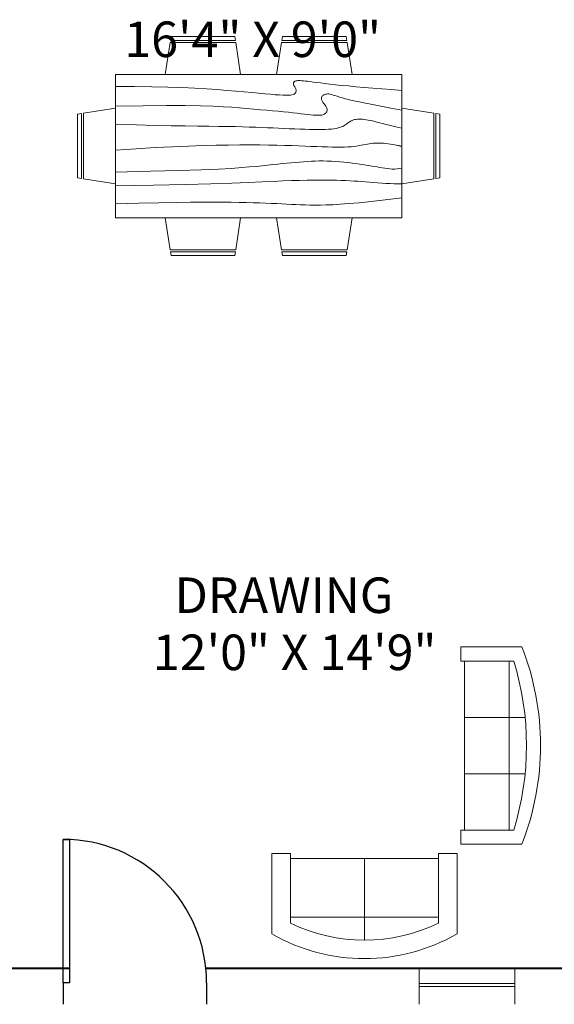
# Model space of a CAD drawing. Units: inches. Extents: x -46 to 1145, y -527 to 760.
# Tile 55 of 57: x 775 to 909, y 222 to 469. Entities that reach past the tile are written whole.
import ezdxf

# ---------------------------------------------------------------- set-up
doc = ezdxf.new("R2010")
doc.units = ezdxf.units.IN
doc.header["$MEASUREMENT"] = 0
for name, color, linetype, lineweight in [('A-AREA-IDEN', 1, 'Continuous', 18), ('A-FURN', 2, 'Continuous', 13), ('DOORS', 3, 'Continuous', 25), ('WALLS', 4, 'Continuous', 40), ('WINDOWS', 240, 'Continuous', 20)]:
    doc.layers.add(name, color=color, linetype=linetype, lineweight=lineweight)
doc.styles.get("Standard").update_dxf_attribs({"font": 'arial.ttf'})

# ---------------------------------------------------------------- blocks, each defined once
blk = doc.blocks.new('Dining Set - 36 x 72 in.')
for p, q in [((-22, 27.5), (-22.1562, 26.50042)), ((-22, 27.5), (-6, 27.5)), ((-5.8437, 26.49966), (-6, 27.5)), ((6, 27.5), (5.8438, 26.50042)), ((6, 27.5), (22, 27.5)), ((22.1563, 26.49966), (22, 27.5)), ((-22.2343, 26.00059), (-23.4847, 17.99762)), ((-22.2304, 26), (-5.7608, 26)), ((-5.8416, 26.5), (-22.1534, 26.5)), ((-4.5152, 17.99762), (-5.7655, 25.99926)), ((5.7657, 26.00059), (4.5153, 17.99762)), ((5.7696, 26), (22.2392, 26)), ((22.1584, 26.5), (5.8466, 26.5)), ((23.4848, 17.99762), (22.2345, 25.99926)), ((36, 18), (-36, 18)), ((-36, 18), (-36, -18)), ((36, -18), (36, 18)), ((-45.5, 8), (-44.5004, 8.15617)), ((-45.5, 8), (-45.5, -8)), ((-44.5, -8.15843), (-44.5, 8.15338)), ((-44.0006, 8.23428), (-35.9976, 9.48474)), ((-44, 8.23041), (-44, -8.23915)), ((44.0006, 8.23428), (35.9976, 9.48474)), ((44, 8.23041), (44, -8.23915)), ((44.5, -8.15843), (44.5, 8.15338)), ((45.5, 8), (44.5005, 8.15617)), ((45.5, 8), (45.5, -8)), ((-44.4997, -8.15631), (-45.5, -8)), ((-35.9976, -9.48476), (-43.9993, -8.2345)), ((35.9976, -9.48476), (43.9993, -8.2345)), ((44.4997, -8.15631), (45.5, -8)), ((-36, -18), (36, -18)), ((-22.2343, -26.0006), (-23.4847, -17.99762)), ((-4.5152, -17.99762), (-5.7655, -25.99928)), ((5.7657, -26.0006), (4.5153, -17.99762)), ((23.4848, -17.99762), (22.2345, -25.99928)), ((-22.2304, -26), (-5.7608, -26)), ((-22, -27.5), (-22.1562, -26.50044)), ((-5.8416, -26.5), (-22.1534, -26.5)), ((-5.8437, -26.49967), (-6, -27.5)), ((5.7696, -26), (22.2392, -26)), ((6, -27.5), (5.8438, -26.50044)), ((22.1584, -26.5), (5.8466, -26.5)), ((22.1563, -26.49967), (22, -27.5)), ((-22, -27.5), (-6, -27.5)), ((6, -27.5), (22, -27.5))]:
    blk.add_line(p, q)
for points in [[(-36, 15), (-31.1772, 14.97754), (-26.8079, 14.91406), (-22.8538, 14.81543), (-19.276, 14.6875), (-16.0362, 14.53613), (-13.0957, 14.36718), (-10.4159, 14.18652), (-7.9583, 14), (-5.6904, 13.81315), (-3.6035, 13.63021), (-1.6954, 13.45508), (0.0365, 13.29166), (1.5945, 13.14388), (2.9811, 13.01562), (4.1988, 12.9108), (5.25, 12.83333), (6.1393, 12.78613), (6.8802, 12.76823), (7.4883, 12.77767), (7.9792, 12.8125), (8.3685, 12.87077), (8.6719, 12.95052), (8.9049, 13.0498), (9.0833, 13.16666), (9.2205, 13.29899), (9.3216, 13.44401), (9.3895, 13.59879), (9.4271, 13.76041), (9.4373, 13.92594), (9.4232, 14.09245), (9.3875, 14.257), (9.3333, 14.41666), (9.2638, 14.56917), (9.1836, 14.71484), (9.0975, 14.85465), (9.0104, 14.98958), (8.9272, 15.1206), (8.8529, 15.2487), (8.7922, 15.37483), (8.75, 15.5), (8.7305, 15.62467), (8.7344, 15.74739), (8.7617, 15.86621), (8.8125, 15.97916), (8.8867, 16.08431), (8.9844, 16.17968), (9.1055, 16.26334), (9.25, 16.33333), (9.4189, 16.38802), (9.6172, 16.42708), (9.8506, 16.45052), (10.125, 16.45833), (10.4463, 16.45052), (10.8203, 16.42708), (11.2529, 16.38802), (11.75, 16.33333), (12.3184, 16.26318), (12.9694, 16.17838), (13.7151, 16.07991), (14.5677, 15.96875), (15.5395, 15.84586), (16.6426, 15.71224), (17.8893, 15.56884), (19.2917, 15.41666), (20.859, 15.25667), (22.5879, 15.08984), (24.4721, 14.91715), (26.5052, 14.73958), (28.6809, 14.5581), (30.9929, 14.3737), (33.4347, 14.18733), (36, 14)], [(-36, 10), (-28.9766, 10.14274), (-23.1725, 10.20442), (-18.4241, 10.19775), (-14.5677, 10.13541), (-11.4399, 10.03011), (-8.877, 9.89453), (-6.7154, 9.74137), (-4.7917, 9.58333), (-2.9698, 9.43082), (-1.2246, 9.28515), (0.4415, 9.14534), (2.026, 9.01041), (3.5266, 8.87939), (4.9408, 8.7513), (6.266, 8.62516), (7.5, 8.5), (8.6411, 8.37549), (9.6914, 8.2539), (10.6538, 8.13818), (11.5312, 8.03125), (12.3267, 7.93603), (13.043, 7.85547), (13.6831, 7.79248), (14.25, 7.75), (14.7471, 7.7303), (15.1797, 7.73307), (15.5537, 7.75732), (15.875, 7.80208), (16.1494, 7.86637), (16.3828, 7.94922), (16.5811, 8.04964), (16.75, 8.16666), (16.8944, 8.29915), (17.0143, 8.44531), (17.1089, 8.60319), (17.1771, 8.77083), (17.218, 8.94629), (17.2305, 9.1276), (17.2137, 9.31282), (17.1667, 9.5), (17.0895, 9.6875), (16.987, 9.875), (16.8649, 10.0625), (16.7292, 10.25), (16.5856, 10.4375), (16.4401, 10.625), (16.2985, 10.8125), (16.1667, 11), (16.05, 11.18733), (15.9518, 11.3737), (15.8752, 11.5581), (15.8229, 11.73958), (15.798, 11.91715), (15.8034, 12.08984), (15.842, 12.25667), (15.9167, 12.41666), (16.0295, 12.56836), (16.1784, 12.70833), (16.3605, 12.83268), (16.5729, 12.9375), (16.8127, 13.01888), (17.0768, 13.07291), (17.3625, 13.0957), (17.6667, 13.08333), (17.9894, 13.03312), (18.3418, 12.94726), (18.7382, 12.82918), (19.1927, 12.68229), (19.7195, 12.51001), (20.3327, 12.31575), (21.0465, 12.10294), (21.875, 11.875), (22.8357, 11.63354), (23.959, 11.37304), (25.2786, 11.08618), (26.8282, 10.76562), (28.6414, 10.40405), (30.752, 9.99414), (33.1936, 9.52856), (36, 9)], [(-36, 5.5), (-30.7157, 5.3348), (-26.069, 5.20963), (-21.9946, 5.11767), (-18.4271, 5.05208), (-15.3009, 5.00602), (-12.5508, 4.97265), (-10.1112, 4.94515), (-7.9167, 4.91666), (-5.909, 4.88167), (-4.0586, 4.83984), (-2.3429, 4.79215), (-0.7396, 4.73958), (0.7739, 4.6831), (2.22, 4.6237), (3.6213, 4.56233), (5, 4.5), (6.373, 4.43782), (7.7344, 4.3776), (9.0723, 4.32129), (10.375, 4.27083), (11.6309, 4.22819), (12.8281, 4.19531), (13.9551, 4.17415), (15, 4.16666), (15.954, 4.17448), (16.819, 4.19791), (17.6001, 4.23698), (18.3021, 4.29166), (18.9299, 4.36198), (19.4883, 4.44791), (19.9823, 4.54948), (20.4167, 4.66666), (20.7969, 4.79899), (21.1302, 4.94401), (21.4245, 5.09879), (21.6875, 5.26041), (21.9271, 5.42594), (22.1511, 5.59245), (22.3672, 5.757), (22.5834, 5.91666), (22.8065, 6.06868), (23.0404, 6.21093), (23.2879, 6.34147), (23.5521, 6.45833), (23.8358, 6.55957), (24.142, 6.64323), (24.4735, 6.70735), (24.8334, 6.75), (25.2235, 6.76969), (25.642, 6.76692), (26.0858, 6.74267), (26.5521, 6.69791), (27.0379, 6.63362), (27.5404, 6.55078), (28.0565, 6.45036), (28.5834, 6.33333), (29.1242, 6.19987), (29.7071, 6.04687), (30.3661, 5.87044), (31.1354, 5.66666), (32.0493, 5.43164), (33.142, 5.16146), (34.4475, 4.85221), (36, 4.5)], [(-36, -1), (-30.7915, -0.6591), (-26.0195, -0.38216), (-21.6519, -0.16284), (-17.6563, 0.00521), (-14.0005, 0.12833), (-10.6523, 0.21289), (-7.5796, 0.26522), (-4.75, 0.29166), (-2.134, 0.29793), (0.2878, 0.28711), (2.5317, 0.26163), (4.6146, 0.22396), (6.5529, 0.17651), (8.3633, 0.12174), (10.0623, 0.06209), (11.6667, 0), (13.1899, -0.06201), (14.6341, -0.1211), (15.9982, -0.17432), (17.2813, -0.21875), (18.4823, -0.25147), (19.6003, -0.26953), (20.6343, -0.27002), (21.5834, -0.25), (22.4481, -0.20768), (23.2357, -0.14584), (23.9549, -0.06836), (24.6146, 0.02083), (25.2235, 0.11784), (25.7904, 0.21875), (26.3241, 0.31966), (26.8334, 0.41666), (27.3265, 0.50618), (27.8099, 0.58593), (28.2894, 0.65397), (28.7709, 0.70833), (29.2601, 0.74707), (29.763, 0.76823), (30.2855, 0.76985), (30.8334, 0.75), (31.4088, 0.70784), (31.9994, 0.64713), (32.589, 0.57275), (33.1615, 0.48958), (33.7008, 0.4025), (34.1908, 0.3164), (34.6153, 0.23616), (34.9584, 0.16666), (35.2099, 0.11165), (35.3848, 0.07031), (35.504, 0.04069), (35.5886, 0.02083), (35.6594, 0.00879), (35.7377, 0.0026), (35.8442, 0.00032), (36, 0)], [(-36, -6.5), (-27.1843, -6.31267), (-20.084, -6.1263), (-14.469, -5.9419), (-10.1094, -5.76042), (-6.7752, -5.58285), (-4.2363, -5.41016), (-2.2629, -5.24333), (-0.625, -5.08334), (0.8708, -4.93099), (2.2715, -4.78646), (3.5872, -4.64974), (4.8281, -4.52084), (6.0046, -4.39974), (7.127, -4.28646), (8.2053, -4.18099), (9.25, -4.08334), (10.2705, -3.99382), (11.2734, -3.91407), (12.2647, -3.84603), (13.25, -3.79167), (14.2354, -3.75293), (15.2266, -3.73177), (16.2295, -3.73015), (17.25, -3.75), (18.2912, -3.79248), (19.3451, -3.85547), (20.4009, -3.93604), (21.4479, -4.03125), (22.4754, -4.13819), (23.4727, -4.25391), (24.4289, -4.37549), (25.3334, -4.5), (26.1785, -4.62492), (26.9694, -4.74935), (27.7145, -4.87281), (28.4219, -4.99479), (29.1, -5.11483), (29.7572, -5.23242), (30.4016, -5.34709), (31.0417, -5.45834), (31.6837, -5.56437), (32.3262, -5.65821), (32.9658, -5.73153), (33.599, -5.77604), (34.2224, -5.78345), (34.8327, -5.74545), (35.4264, -5.65373), (36, -5.5)], [(-36, -10), (-26.4022, -9.81299), (-18.4675, -9.62891), (-11.9839, -9.45069), (-6.7396, -9.28125), (-2.5226, -9.12354), (0.8789, -8.98047), (3.6769, -8.85498), (6.0833, -8.75), (8.2767, -8.66765), (10.3021, -8.60677), (12.1712, -8.56543), (13.8958, -8.54167), (15.4876, -8.53353), (16.9583, -8.53907), (18.3197, -8.55632), (19.5834, -8.58334), (20.7616, -8.61841), (21.8685, -8.66081), (22.9188, -8.71004), (23.9271, -8.76563), (24.9081, -8.82707), (25.8763, -8.89388), (26.8465, -8.96558), (27.8334, -9.04167), (28.8474, -9.12118), (29.8828, -9.20117), (30.93, -9.27824), (31.9792, -9.34896), (33.0205, -9.40991), (34.0443, -9.45768), (35.0407, -9.48885), (36, -9.5)], [(-36, -14.5), (-30.0881, -14.33513), (-25.0332, -14.21224), (-20.7312, -14.12647), (-17.0781, -14.07292), (-13.97, -14.04671), (-11.3027, -14.04297), (-8.9724, -14.05681), (-6.875, -14.08334), (-4.9224, -14.11833), (-3.0905, -14.16016), (-1.3709, -14.20785), (0.2448, -14.26042), (1.7647, -14.3169), (3.1973, -14.3763), (4.5507, -14.43767), (5.8333, -14.5), (7.0554, -14.5621), (8.235, -14.62175), (9.3922, -14.67652), (10.5469, -14.72396), (11.7192, -14.76164), (12.929, -14.78711), (14.1965, -14.79794), (15.5417, -14.79167), (16.9933, -14.76424), (18.6152, -14.70508), (20.4804, -14.60197), (22.6615, -14.44271), (25.2312, -14.21509), (28.2624, -13.9069), (31.8277, -13.50594), (36, -13)]]:
    blk.add_lwpolyline(points)
blk = doc.blocks.new('Sofa - Roundback 7 ft.')
for p, q in [((-12.00002, -32.4421), (-12.00003, -6.5971)), ((11.99997, -32.4421), (11.99998, -6.5971)), ((-36.000027, -34), (-36.000027, -11.4696)), ((35.99998, -34), (35.99998, -11.4696)), ((-35.999844, -13.3819), (35.9998, -13.3819)), ((-36.000027, -32.4421), (35.99998, -32.4421))]:
    blk.add_line(p, q)
for points in [[(-36.000027, -34), (-42.000027, -34), (-42.000027, -8)], [(41.99998, -8), (41.99998, -34), (35.99998, -34)]]:
    blk.add_lwpolyline(points)
for centre, radius, start, end in [((0, -114.25), 114.25, 68.43141, 111.5686), ((-0.00001, -127.1968), 121.1968, 72.72033, 107.2797)]:
    blk.add_arc(centre, radius, start, end)
blk = doc.blocks.new('Sofa - Roundback Loveseat 5 ft.')
for p, q in [((0, -32.44198), (0, -5.99998)), ((-24, -33.99998), (-24, -11.46958)), ((24.00004, -33.99998), (24.00004, -11.46958)), ((-23.9998, -13.38178), (23.99986, -13.38178)), ((-24, -32.44198), (24.00004, -32.44198))]:
    blk.add_line(p, q)
for points in [[(-24, -33.99998), (-30, -33.99998), (-30, -7.99998)], [(30.00004, -7.99998), (30.00004, -33.99998), (24.00004, -33.99998)]]:
    blk.add_lwpolyline(points)
for centre, radius, start, end in [((0, -60.24998), 60.24998, 60.13715, 119.8628), ((0, -61.38438), 55.38444, 64.32083, 115.6792)]:
    blk.add_arc(centre, radius, start, end)
blk = doc.blocks.new('*U2')
for p, q in [((0, 0), (0, -6)), ((40, 0), (40, -6))]:
    blk.add_line(p, q)
blk.add_lwpolyline([(0, 0), (0, 40), (1.75, 40), (1.75, 0)], close=True)
blk.add_arc((0, 0), 40, 0, 90)
blk = doc.blocks.new('WINDOW-24IN')
for p, q in [((0, 4.5), (0, 9)), ((0, 9), (0, 0)), ((24, 9), (24, 0)), ((0, 5.23), (24, 5.23)), ((0, 4.5), (24, 4.5))]:
    blk.add_line(p, q)

msp = doc.modelspace()

# ---------------------------------------------------------------- linework, layer by layer
at = {"layer": 'WALLS'}
for p, q in [((787.3481, 230.5176), (767.0637, 230.5176)), ((911.0637, 230.5176), (821.5926, 230.5176))]:
    msp.add_line(p, q, dxfattribs=at)

# ---------------------------------------------------------------- block references
at = {"layer": 'A-FURN'}
msp.add_blockref('Dining Set - 36 x 72 in.', (834.8617, 436.9572), dxfattribs=at)
for name, p, xscale, yscale, zscale, rotation in [('Sofa - Roundback 7 ft.', (905.7179, 286.4838), 0.5892128430585409, 0.5892128430585409, 0.5892128430585409, 270), ('Sofa - Roundback Loveseat 5 ft.', (861.4562, 232.9861), 0.7756934806711657, 0.7756934806711657, 0.7756934806711657, 180)]:
    msp.add_blockref(name, p, dxfattribs=dict(at, xscale=xscale, yscale=yscale, zscale=zscale, rotation=rotation))
at = {"layer": 'DOORS', "xscale": 0.9, "yscale": 0.9, "zscale": 0.9}
msp.add_blockref('*U2', (785.7731, 226.9176), dxfattribs=at)
at = {"layer": 'WINDOWS'}
msp.add_blockref('WINDOW-24IN', (875.233, 221.518), dxfattribs=at)

# ---------------------------------------------------------------- texts
at = {"layer": 'A-AREA-IDEN'}
for s, height, p in [('16\'4" X 9\'0"', 8.923264, (801.1059, 459.3065)), ('  DRAWING', 8.92326, (808.2854, 319.7456)), ('12\'0" X 14\'9"', 8.923264, (808.2854, 305.4112))]:
    msp.add_text(s, height=height, dxfattribs=at).set_placement(p)

doc.saveas('drawing.dxf')
